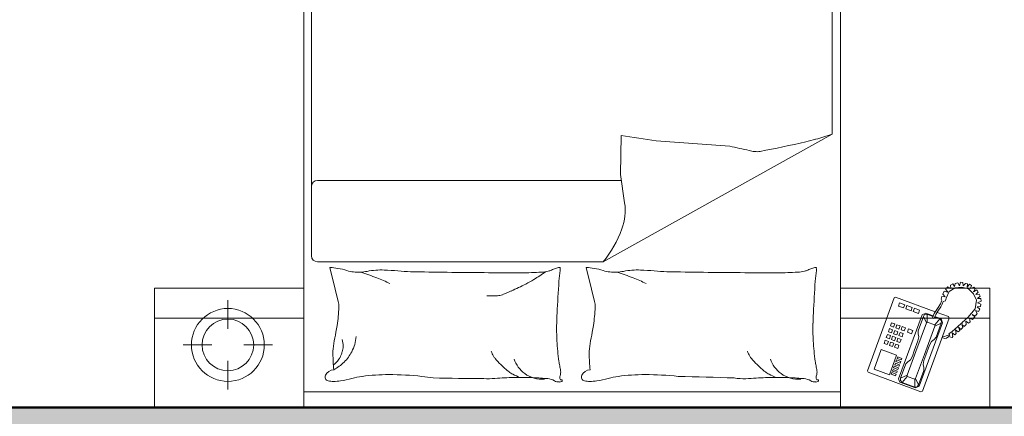
# Model space of a CAD drawing. Units: inches. Extents: x -7 to 1228, y -146 to 1091.
# Tile 60 of 88: x 429 to 531, y 573 to 614. Entities that reach past the tile are written whole.
import ezdxf

# ---------------------------------------------------------------- set-up
doc = ezdxf.new("R2010")
doc.units = ezdxf.units.IN
for name, color, linetype, lineweight in [('A-FURN', 8, 'Continuous', 18), ('A-WALL', 7, 'Continuous', 50), ('A-WALL-PATT', 251, 'Continuous', 13)]:
    doc.layers.add(name, color=color, linetype=linetype, lineweight=lineweight)
doc.styles.add('DIM_FONT', font='SIMPLEX.shx', dxfattribs={"width": 0.8})

# ---------------------------------------------------------------- blocks, each defined once
blk = doc.blocks.new('A$C4F634EDD')
for p, q in [((0, 2.6295), (0, 2.2295)), ((0.5, 2.6295), (0, 2.6295)), ((0.5, 2.6295), (2.3, 2.6295)), ((0.5, 0.5295), (0.5, 2.6295)), ((0.5, 2.2295), (0.5, 2.6295)), ((2.3, 2.6295), (2.3, 0.5295)), ((2.3, 2.6295), (2.8, 2.6295)), ((2.3, 2.2295), (2.3, 2.6295)), ((2.8, 2.6295), (2.8, 2.2295)), ((0.5, 2.5771), (2.3, 2.5771)), ((2.392, 2.5115), (2.5692, 2.5765)), ((2.5692, 2.5765), (2.574, 2.5743)), ((0.2457, 2.5697), (0.2457, 2.4733)), ((2.4946, 2.5331), (2.4985, 2.5445)), ((2.4985, 2.5445), (2.5516, 2.564)), ((2.5062, 2.5454), (2.5004, 2.5392)), ((2.5062, 2.5454), (2.5487, 2.561)), ((2.5235, 2.5256), (2.5062, 2.5454)), ((2.5483, 2.5347), (2.5487, 2.561)), ((2.5487, 2.561), (2.5571, 2.56)), ((2.5615, 2.5536), (2.5514, 2.5318)), ((2.5516, 2.564), (2.5637, 2.5584)), ((2.5571, 2.56), (2.5615, 2.5536)), ((2.5615, 2.5536), (2.5791, 2.5058)), ((2.5637, 2.5584), (2.6418, 2.3458)), ((2.574, 2.5743), (2.6638, 2.3298)), ((2.3898, 2.5066), (2.392, 2.5115)), ((2.412, 2.5007), (2.4634, 2.5196)), ((2.4634, 2.5196), (2.4875, 2.454)), ((2.4842, 2.5232), (2.47, 2.518)), ((2.47, 2.518), (2.472, 2.5127)), ((2.472, 2.5127), (2.4862, 2.5179)), ((2.4881, 2.5126), (2.4739, 2.5074)), ((2.4862, 2.5179), (2.4842, 2.5232)), ((2.4901, 2.5073), (2.4881, 2.5126)), ((2.5734, 2.3187), (2.4946, 2.5331)), ((2.5004, 2.5392), (2.5013, 2.5315)), ((2.5013, 2.5315), (2.5188, 2.4836)), ((2.5013, 2.5315), (2.5231, 2.5214)), ((2.5231, 2.5214), (2.5235, 2.5256)), ((2.5523, 2.4417), (2.5231, 2.5214)), ((2.5483, 2.5347), (2.5235, 2.5256)), ((2.5514, 2.5318), (2.5483, 2.5347)), ((2.5807, 2.4521), (2.5514, 2.5318)), ((2.4795, 2.2621), (2.3898, 2.5066)), ((2.4361, 2.4352), (2.412, 2.5007)), ((2.4739, 2.5074), (2.4759, 2.502)), ((2.4759, 2.502), (2.4901, 2.5073)), ((2.492, 2.5019), (2.4778, 2.4967)), ((2.4778, 2.4967), (2.4798, 2.4914)), ((2.4798, 2.4914), (2.494, 2.4966)), ((2.4959, 2.4913), (2.4817, 2.4861)), ((2.4817, 2.4861), (2.4837, 2.4808)), ((2.4837, 2.4808), (2.4979, 2.486)), ((2.4998, 2.4807), (2.4856, 2.4755)), ((2.494, 2.4966), (2.492, 2.5019)), ((2.4979, 2.486), (2.4959, 2.4913)), ((2.5018, 2.4754), (2.4998, 2.4807)), ((2.5188, 2.4836), (2.5256, 2.4761)), ((2.5256, 2.4761), (2.5342, 2.4692)), ((2.5788, 2.4956), (2.5767, 2.4848)), ((2.5767, 2.4848), (2.5795, 2.4717)), ((2.5791, 2.5058), (2.5788, 2.4956)), ((2.4875, 2.454), (2.4361, 2.4352)), ((2.4856, 2.4755), (2.4876, 2.4702)), ((2.4876, 2.4702), (2.5018, 2.4754)), ((2.5037, 2.47), (2.4895, 2.4648)), ((2.4895, 2.4648), (2.4915, 2.4595)), ((2.4915, 2.4595), (2.5057, 2.4647)), ((2.5057, 2.4647), (2.5037, 2.47)), ((2.5342, 2.4692), (2.5405, 2.4574)), ((2.5405, 2.4574), (2.547, 2.4397)), ((2.5795, 2.4717), (2.586, 2.454)), ((2.5807, 2.4521), (2.6158, 2.3564)), ((2.5984, 2.4204), (2.586, 2.454)), ((0.0957, 2.4197), (0.192, 2.4197)), ((0.2994, 2.4197), (0.3957, 2.4197)), ((2.4457, 2.4146), (2.4563, 2.4185)), ((2.4496, 2.4039), (2.4457, 2.4146)), ((2.4563, 2.4185), (2.4602, 2.4078)), ((2.4634, 2.4211), (2.474, 2.425)), ((2.4673, 2.4104), (2.4634, 2.4211)), ((2.4779, 2.4143), (2.4673, 2.4104)), ((2.474, 2.425), (2.4779, 2.4143)), ((2.4811, 2.4276), (2.4917, 2.4315)), ((2.485, 2.4169), (2.4811, 2.4276)), ((2.4956, 2.4208), (2.485, 2.4169)), ((2.4883, 2.4081), (2.4989, 2.412)), ((2.4917, 2.4315), (2.4956, 2.4208)), ((2.4989, 2.412), (2.5028, 2.4014)), ((2.5594, 2.4061), (2.547, 2.4397)), ((2.5523, 2.4417), (2.5875, 2.346)), ((2.6047, 2.4086), (2.5984, 2.4204)), ((2.4602, 2.4078), (2.4496, 2.4039)), ((2.4528, 2.3951), (2.4635, 2.399)), ((2.4567, 2.3844), (2.4528, 2.3951)), ((2.4674, 2.3883), (2.4567, 2.3844)), ((2.46, 2.3756), (2.4706, 2.3795)), ((2.4635, 2.399), (2.4674, 2.3883)), ((2.4706, 2.4016), (2.4812, 2.4055)), ((2.4745, 2.3909), (2.4706, 2.4016)), ((2.4706, 2.3795), (2.4745, 2.3689)), ((2.4851, 2.3949), (2.4745, 2.3909)), ((2.4777, 2.3821), (2.4883, 2.386)), ((2.4816, 2.3715), (2.4777, 2.3821)), ((2.4812, 2.4055), (2.4851, 2.3949)), ((2.4922, 2.3975), (2.4883, 2.4081)), ((2.4883, 2.386), (2.4922, 2.3754)), ((2.5028, 2.4014), (2.4922, 2.3975)), ((2.4954, 2.3886), (2.5061, 2.3925)), ((2.4993, 2.378), (2.4954, 2.3886)), ((2.51, 2.3819), (2.4993, 2.378)), ((2.5061, 2.3925), (2.51, 2.3819)), ((2.5238, 2.3769), (2.538, 2.3821)), ((2.5277, 2.3663), (2.5238, 2.3769)), ((2.538, 2.3821), (2.5419, 2.3715)), ((2.5622, 2.393), (2.5594, 2.4061)), ((2.5598, 2.372), (2.5601, 2.3822)), ((2.5601, 2.3822), (2.5622, 2.393)), ((2.6133, 2.4017), (2.6047, 2.4086)), ((2.6201, 2.3941), (2.6133, 2.4017)), ((2.6376, 2.3463), (2.6201, 2.3941)), ((2.6499, 2.3979), (2.6397, 2.3953)), ((2.6417, 2.39), (2.6488, 2.391)), ((2.6488, 2.391), (2.6538, 2.3895)), ((2.6551, 2.397), (2.6499, 2.3979)), ((2.6538, 2.3895), (2.6596, 2.388)), ((2.6627, 2.392), (2.6551, 2.397)), ((2.6596, 2.388), (2.6626, 2.3867)), ((2.6626, 2.3867), (2.6662, 2.388)), ((2.6692, 2.394), (2.6627, 2.392)), ((2.6662, 2.388), (2.6632, 2.3828)), ((2.6632, 2.3828), (2.6736, 2.3744)), ((2.6736, 2.3944), (2.6692, 2.394)), ((2.6765, 2.391), (2.6736, 2.3944)), ((2.6742, 2.3795), (2.6765, 2.391)), ((2.6824, 2.3858), (2.6742, 2.3795)), ((2.6873, 2.3815), (2.6824, 2.3858)), ((2.6853, 2.369), (2.6873, 2.3815)), ((0.2457, 2.366), (0.2457, 2.2697)), ((2.4639, 2.365), (2.46, 2.3756)), ((2.4745, 2.3689), (2.4639, 2.365)), ((2.4672, 2.3561), (2.4778, 2.36)), ((2.4711, 2.3455), (2.4672, 2.3561)), ((2.4817, 2.3494), (2.4711, 2.3455)), ((2.4778, 2.36), (2.4817, 2.3494)), ((2.4922, 2.3754), (2.4816, 2.3715)), ((2.4849, 2.3626), (2.4955, 2.3665)), ((2.4888, 2.352), (2.4849, 2.3626)), ((2.4994, 2.3559), (2.4888, 2.352)), ((2.4955, 2.3665), (2.4994, 2.3559)), ((2.5026, 2.3691), (2.5132, 2.373)), ((2.5065, 2.3585), (2.5026, 2.3691)), ((2.5171, 2.3624), (2.5065, 2.3585)), ((2.5132, 2.373), (2.5171, 2.3624)), ((2.5419, 2.3715), (2.5277, 2.3663)), ((2.5774, 2.3242), (2.5598, 2.372)), ((2.5774, 2.3242), (2.5875, 2.346)), ((2.5875, 2.346), (2.5905, 2.3431)), ((2.6154, 2.3522), (2.5905, 2.3431)), ((2.6158, 2.3564), (2.6154, 2.3522)), ((2.6154, 2.3522), (2.6327, 2.3324)), ((2.6376, 2.3463), (2.6158, 2.3564)), ((2.6418, 2.3458), (2.6369, 2.332)), ((2.6385, 2.3386), (2.6376, 2.3463)), ((2.6736, 2.3744), (2.6922, 2.3593)), ((2.6946, 2.376), (2.6853, 2.369)), ((2.6922, 2.3593), (2.7051, 2.3473)), ((2.6995, 2.3713), (2.6946, 2.376)), ((2.695, 2.3603), (2.6995, 2.3713)), ((2.7031, 2.3682), (2.695, 2.3603)), ((2.7096, 2.3616), (2.7031, 2.3682)), ((2.7051, 2.3473), (2.7079, 2.3475)), ((2.7062, 2.351), (2.7096, 2.3616)), ((2.7147, 2.3578), (2.7062, 2.351)), ((2.7079, 2.3475), (2.7079, 2.3443)), ((2.7079, 2.3443), (2.727, 2.3277)), ((2.7214, 2.3517), (2.7147, 2.3578)), ((2.7196, 2.34), (2.7214, 2.3517)), ((2.7286, 2.3466), (2.7196, 2.34)), ((2.7346, 2.3423), (2.7286, 2.3466)), ((0, 2.3301), (0.5, 2.3301)), ((2.8, 2.3301), (2.3, 2.3301)), ((2.561, 2.3141), (2.5433, 2.3076)), ((2.5649, 2.3035), (2.561, 2.3141)), ((2.5855, 2.3131), (2.5734, 2.3187)), ((2.5818, 2.3178), (2.5774, 2.3242)), ((2.5901, 2.3168), (2.5818, 2.3178)), ((2.6104, 2.3222), (2.5855, 2.3131)), ((2.5905, 2.3431), (2.5901, 2.3168)), ((2.5901, 2.3168), (2.6097, 2.324)), ((2.613, 2.3312), (2.6077, 2.3293)), ((2.6077, 2.3293), (2.6135, 2.3141)), ((2.6192, 2.3174), (2.613, 2.3312)), ((2.6135, 2.3141), (2.6244, 2.2977)), ((2.6153, 2.3261), (2.6327, 2.3324)), ((2.6369, 2.332), (2.6161, 2.3243)), ((2.626, 2.3069), (2.6192, 2.3174)), ((2.6616, 2.3249), (2.6234, 2.3109)), ((2.6327, 2.3324), (2.6385, 2.3386)), ((2.6638, 2.3298), (2.6616, 2.3249)), ((2.727, 2.3277), (2.7512, 2.2983)), ((2.732, 2.3295), (2.7346, 2.3423)), ((2.7423, 2.3345), (2.732, 2.3295)), ((2.7406, 2.3172), (2.7495, 2.325)), ((2.7519, 2.3218), (2.7406, 2.3172)), ((2.7495, 2.325), (2.7423, 2.3345)), ((2.7575, 2.3144), (2.7519, 2.3218)), ((2.7526, 2.3045), (2.7575, 2.3144)), ((2.6172, 2.3086), (2.4844, 2.2599)), ((2.5114, 2.2959), (2.4936, 2.2894)), ((2.4936, 2.2894), (2.4976, 2.2788)), ((2.4976, 2.2788), (2.5153, 2.2853)), ((2.5153, 2.2853), (2.5114, 2.2959)), ((2.5362, 2.305), (2.5185, 2.2985)), ((2.5185, 2.2985), (2.5224, 2.2879)), ((2.5224, 2.2879), (2.5401, 2.2944)), ((2.5401, 2.2944), (2.5362, 2.305)), ((2.5433, 2.3076), (2.5472, 2.297)), ((2.5472, 2.297), (2.5649, 2.3035)), ((2.6244, 2.2977), (2.6349, 2.2825)), ((2.6365, 2.2916), (2.626, 2.3069)), ((2.6349, 2.2825), (2.638, 2.273)), ((2.6407, 2.2834), (2.6365, 2.2916)), ((2.6438, 2.2739), (2.6407, 2.2834)), ((2.7512, 2.2983), (2.756, 2.2695)), ((2.7622, 2.308), (2.7526, 2.3045)), ((2.7574, 2.2924), (2.7673, 2.2997)), ((2.7687, 2.2905), (2.7574, 2.2924)), ((2.7587, 2.279), (2.7699, 2.2828)), ((2.7708, 2.2725), (2.7587, 2.279)), ((2.7673, 2.2997), (2.7622, 2.308)), ((2.7699, 2.2828), (2.7687, 2.2905)), ((0.5953, 2.1912), (0.616, 2.2738)), ((1.4546, 2.1912), (1.4752, 2.2738)), ((2.4844, 2.2599), (2.4795, 2.2621)), ((2.6399, 2.2712), (2.6374, 2.2659)), ((2.6374, 2.2659), (2.6398, 2.257)), ((2.638, 2.273), (2.6399, 2.2712)), ((2.6398, 2.257), (2.6509, 2.259)), ((2.6509, 2.259), (2.6431, 2.2492)), ((2.6431, 2.2492), (2.6473, 2.2398)), ((2.6519, 2.2716), (2.6438, 2.2739)), ((2.6535, 2.2628), (2.6519, 2.2716)), ((2.6636, 2.2409), (2.6535, 2.2628)), ((2.7459, 2.2483), (2.7284, 2.2317)), ((2.756, 2.2695), (2.7459, 2.2483)), ((2.7529, 2.2505), (2.7645, 2.2498)), ((2.7607, 2.2424), (2.7529, 2.2505)), ((2.759, 2.2637), (2.7706, 2.2643)), ((2.7676, 2.2559), (2.759, 2.2637)), ((2.7645, 2.2498), (2.7676, 2.2559)), ((2.7706, 2.2643), (2.7708, 2.2725)), ((0, 2.2295), (0.5, 2.2295)), ((2.8, 2.2295), (2.3, 2.2295)), ((2.6473, 2.2398), (2.6592, 2.2429)), ((2.6592, 2.2429), (2.6521, 2.2314)), ((2.6521, 2.2314), (2.6598, 2.2248)), ((2.6598, 2.2248), (2.6697, 2.2309)), ((2.6836, 2.2287), (2.6636, 2.2409)), ((2.6697, 2.2309), (2.6684, 2.219)), ((2.6684, 2.219), (2.6761, 2.2145)), ((2.6761, 2.2145), (2.6821, 2.2237)), ((2.6821, 2.2237), (2.6843, 2.2135)), ((2.7063, 2.2256), (2.6836, 2.2287)), ((2.6843, 2.2135), (2.6927, 2.2117)), ((2.6927, 2.2117), (2.6986, 2.222)), ((2.6986, 2.222), (2.7019, 2.2098)), ((2.7284, 2.2317), (2.7063, 2.2256)), ((2.7102, 2.2104), (2.7113, 2.2218)), ((2.7113, 2.2218), (2.7192, 2.2137)), ((2.7192, 2.2137), (2.7255, 2.2152)), ((2.7255, 2.2152), (2.7242, 2.2265)), ((2.7242, 2.2265), (2.7324, 2.2165)), ((2.7324, 2.2165), (2.7386, 2.2208)), ((2.7386, 2.2208), (2.7354, 2.2306)), ((2.7354, 2.2306), (2.7462, 2.2264)), ((2.7509, 2.2314), (2.7459, 2.2418)), ((2.7459, 2.2418), (2.7568, 2.2352)), ((2.7462, 2.2264), (2.7509, 2.2314)), ((2.7568, 2.2352), (2.7607, 2.2424)), ((0.5878, 2.1612), (0.5953, 2.1912)), ((1.4471, 2.1612), (1.4546, 2.1912)), ((2.7019, 2.2098), (2.7102, 2.2104)), ((0.5258, 2.121), (0.5258, 0.5617)), ((1.5035, 2.141), (0.5458, 2.141)), ((1.5035, 2.141), (2.2716, 1.7136)), ((1.576, 1.9433), (1.5624, 1.8479)), ((0.5458, 1.8684), (1.5653, 1.8684)), ((1.5624, 1.8479), (1.5641, 1.7178)), ((2.2716, 0.5617), (2.2716, 1.7136))]:
    blk.add_line(p, q)
for radius in [0.1222, 0.0865]:
    blk.add_circle((0.2457, 2.4197), radius)
for centre, radius, start, end in [((0.5999, 2.4516), 0.0904, 90, 101.2724), ((0.5999, 2.3808), 0.1611, 81.5628, 90), ((1.3554, 2.5152), 0.0289, 85.6975, 120.6513), ((1.3556, 2.519), 0.0251, 68.2117, 85.6975), ((1.3637, 2.5391), 0.00342, 19.564, 68.2117), ((1.4591, 2.4516), 0.0904, 90, 101.2724), ((1.4591, 2.3808), 0.1611, 81.5628, 90), ((2.2146, 2.5152), 0.0289, 85.6975, 120.6513), ((2.2149, 2.519), 0.0251, 68.2117, 85.6975), ((2.2229, 2.5391), 0.00342, 19.564, 68.2117), ((0.5848, 2.5274), 0.0131, 101.2724, 206.5805), ((0.6036, 2.5368), 0.0342, 206.5805, 265.5998), ((0.5788, 2.2388), 0.3048, 74.256, 81.5628), ((0.7272, 2.7653), 0.2422, 254.256, 262.4531), ((0.7851, 3.2019), 0.6827, 262.4531, 270), ((0.7851, 3.5682), 1.049, 270, 276.0867), ((0.8402, 3.0514), 0.5293, 276.0867, 280.1899), ((1.1602, -8.1346), 10.6675, 90.30153, 91.21582), ((1.1169, 2.2433), 0.2897, 85.1982, 92.5386), ((1.2142, 3.4021), 0.8732, 265.1982, 269.4243), ((1.4317, 2.2032), 0.3916, 128.3886, 133.8115), ((1.2362, 2.45), 0.0768, 117.2396, 128.3886), ((1.3082, 2.3102), 0.234, 110.8603, 117.2396), ((1.2204, 4.0232), 1.4943, 269.4243, 271.9079), ((1.2995, 2.4357), 0.0992, 126.0864, 143.8234), ((1.2995, 2.4357), 0.0992, 105.9352, 126.0864), ((1.2429, 3.3501), 0.8208, 271.9079, 275.2592), ((1.2995, 2.4357), 0.0992, 85.7841, 105.9352), ((1.3132, 2.5864), 0.0539, 275.2592, 300.6513), ((1.3739, 2.5288), 0.0156, 158.0096, 201.421), ((1.3634, 2.533), 0.00428, 78.1069, 158.0096), ((1.3288, 2.5111), 0.0328, 351.8665, 21.421), ((1.3647, 2.5395), 0.00232, 258.1069, 19.564), ((1.444, 2.5274), 0.0131, 101.2724, 206.5805), ((1.4628, 2.5368), 0.0342, 206.5805, 265.5998), ((1.438, 2.2388), 0.3048, 74.256, 81.5628), ((1.5865, 2.7653), 0.2422, 254.256, 262.4531), ((1.6443, 3.2019), 0.6827, 262.4531, 270), ((1.6443, 3.5682), 1.049, 270, 276.0867), ((1.4785, 15.4878), 12.9656, 271.22425, 272.05324), ((1.97, 2.3805), 0.1524, 92.5386, 100.1899), ((1.9761, 2.2433), 0.2897, 85.1982, 92.5386), ((2.0734, 3.4021), 0.8732, 265.1982, 269.4243), ((2.291, 2.2032), 0.3916, 128.3886, 133.8115), ((2.0954, 2.45), 0.0768, 117.2396, 128.3886), ((2.1674, 2.3102), 0.234, 110.8603, 117.2396), ((2.0797, 4.0232), 1.4943, 269.4243, 271.9079), ((2.1588, 2.4357), 0.0992, 126.0864, 143.8234), ((2.1588, 2.4357), 0.0992, 105.9352, 126.0864), ((2.1021, 3.3501), 0.8208, 271.9079, 275.2592), ((2.1588, 2.4357), 0.0992, 85.7841, 105.9352), ((2.1724, 2.5864), 0.0539, 275.2592, 300.6513), ((2.2331, 2.5288), 0.0156, 158.0096, 201.421), ((2.2226, 2.533), 0.00428, 78.1069, 158.0096), ((2.1881, 2.5111), 0.0328, 351.8665, 21.421), ((2.224, 2.5395), 0.00232, 258.1069, 19.564), ((1.0898, 2.4496), 0.4918, 173.7676, 180), ((0.5462, 2.4142), 0.0899, 41.4429, 53.7359), ((0.5368, 2.3783), 0.1399, 45.0976, 62.7964), ((0.5368, 2.3783), 0.1399, 27.3988, 45.0976), ((1.3165, 2.3233), 0.2252, 133.8115, 140.9651), ((1.2995, 2.4357), 0.0992, 143.8234, 161.5603), ((1.5522, 2.448), 0.1983, 167.8905, 172.3191), ((1.1177, 2.5413), 0.246, 347.8905, 351.8665), ((1.949, 2.4496), 0.4918, 173.7676, 180), ((2.1757, 2.3233), 0.2252, 133.8115, 140.9651), ((2.1588, 2.4357), 0.0992, 143.8234, 161.5603), ((2.4114, 2.448), 0.1983, 167.8905, 172.3191), ((1.977, 2.5413), 0.246, 347.8905, 351.8665), ((0.8019, 2.4496), 0.204, 180, 189.6844), ((0.5741, 2.4389), 0.0526, 25.3551, 41.4429), ((0.4851, 2.3967), 0.1511, 21.8149, 25.3551), ((0.4345, 2.3765), 0.2056, 18.7799, 21.8149), ((1.3127, 2.3625), 0.2002, 151.6832, 156.9972), ((1.1799, 2.4341), 0.0493, 140.9651, 151.6832), ((2.2605, 2.3525), 0.9131, 172.3191, 176.6313), ((1.6611, 2.4496), 0.204, 180, 189.6844), ((2.1719, 2.3625), 0.2002, 151.6832, 156.9972), ((2.0391, 2.4341), 0.0493, 140.9651, 151.6832), ((3.1198, 2.3525), 0.9131, 172.3191, 176.6313), ((1.4703, 2.5637), 0.882, 189.6844, 192.1984), ((0.576, 2.4246), 0.0562, 0, 18.7799), ((0.5406, 2.4246), 0.0915, 345.3149, 0), ((0.5368, 2.3783), 0.1399, 16.515, 27.3988), ((0.5368, 2.3783), 0.1399, 5.6311, 16.515), ((2.3295, 2.5637), 0.882, 189.6844, 192.1984), ((0.2982, 2.3103), 0.3171, 8.0051, 12.1984), ((2.0266, 2.3663), 0.6787, 176.6313, 181.6331), ((1.1575, 2.3103), 0.3171, 8.0051, 12.1984), ((2.8858, 2.3663), 0.6787, 176.6313, 181.6331), ((-0.0401, 2.2627), 0.6588, 2.6649, 8.0051), ((2.7128, 2.3859), 1.3652, 181.6331, 183.055), ((0.8191, 2.2627), 0.6588, 2.6649, 8.0051), ((3.5721, 2.3859), 1.3652, 181.6331, 183.055), ((14.9657, 3.0398), 13.6356, 183.05496, 183.50486), ((15.8249, 3.0398), 13.6356, 183.05496, 183.50486), ((0.5503, 2.2902), 0.0677, 345.9548, 2.6649), ((1.4096, 2.2902), 0.0677, 345.9548, 2.6649), ((1.1303, 1.9835), 0.2721, 85.9172, 93.5552), ((1.1455, 2.197), 0.058, 69.3257, 85.9172), ((0.9871, 1.7772), 0.5066, 65.6735, 69.3257), ((0.473, 2.8815), 0.7387, 293.4844, 295.3111), ((0.6058, 0.9338), 1.4323, 63.5015, 65.6735), ((1.1054, 1.9358), 0.3126, 57.865, 63.5015), ((1.3322, 2.8815), 0.7387, 293.4844, 295.3111), ((0.473, 2.8815), 0.7387, 287.1982, 289.428), ((0.473, 2.8815), 0.7387, 289.428, 291.6577), ((0.473, 2.8815), 0.7387, 291.6577, 293.4844), ((0.8841, 1.5835), 0.7286, 54.1737, 57.865), ((1.6762, 2.2258), 0.3212, 183.5049, 189.9984), ((1.3322, 2.8815), 0.7387, 287.1982, 289.428), ((1.3322, 2.8815), 0.7387, 289.428, 291.6577), ((1.3322, 2.8815), 0.7387, 291.6577, 293.4844), ((2.5355, 2.2258), 0.3212, 183.5049, 189.9984), ((0.5887, 2.1609), 0.000917, 165.9551, 274.0829), ((0.5695, 2.4301), 0.2708, 274.0829, 279.4841), ((0.5763, 2.3896), 0.2297, 279.4841, 287.3864), ((0.6807, 2.0561), 0.1197, 96.4341, 107.3864), ((0.6836, 2.0301), 0.1459, 78.4414, 96.4341), ((0.759, 2.3985), 0.2301, 258.4414, 272.7491), ((0.7026, 3.5718), 1.4048, 272.7491, 274.6176), ((0.9136, 0.9591), 1.2165, 92.6096, 94.6176), ((1.2501, -19.8405), 22.0183, 90.37908, 91.01965), ((1.2012, -3.5404), 5.7185, 89.7135, 90.9704), ((1.224, 1.0141), 1.164, 86.426, 89.7135), ((1.2875, 2.0302), 0.1459, 77.131, 86.426), ((1.3099, 2.1283), 0.0453, 62.7159, 77.131), ((1.3658, 2.2367), 0.0767, 242.7159, 253.7788), ((1.3688, 2.247), 0.0875, 253.7788, 262.8796), ((1.3581, 2.1615), 0.00132, 262.8796, 343.3022), ((1.3409, 2.1667), 0.0193, 343.3022, 9.9984), ((1.448, 2.1609), 0.000917, 165.9551, 274.0829), ((1.4288, 2.4301), 0.2708, 274.0829, 279.4841), ((1.4355, 2.3896), 0.2297, 279.4841, 287.3864), ((1.5399, 2.0561), 0.1197, 96.4341, 107.3864), ((1.5429, 2.0301), 0.1459, 78.4414, 96.4341), ((1.6182, 2.3985), 0.2301, 258.4414, 272.7491), ((1.5619, 3.5718), 1.4048, 272.7491, 274.6176), ((1.7729, 0.9591), 1.2165, 92.6096, 94.6176), ((2.1093, -19.8405), 22.0183, 90.37908, 91.01965), ((2.0605, -3.5404), 5.7185, 89.7135, 90.9704), ((2.0833, 1.0141), 1.164, 86.426, 89.7135), ((2.1467, 2.0302), 0.1459, 77.131, 86.426), ((2.1691, 2.1283), 0.0453, 62.7159, 77.131), ((2.2251, 2.2367), 0.0767, 242.7159, 253.7788), ((2.2281, 2.247), 0.0875, 253.7788, 262.8796), ((2.2174, 2.1615), 0.00132, 262.8796, 343.3022), ((2.2001, 2.1667), 0.0193, 343.3022, 9.9984), ((0.5458, 2.121), 0.02, 90, 180), ((1.2147, 1.9017), 0.3751, 20.1488, 39.6445), ((1.3977, 1.9688), 0.1801, 351.8644, 20.1488), ((0.5458, 1.8884), 0.02, 180, 270), ((0.6102, 18.0525), 16.3521, 273.75703, 274.62393), ((1.4194, 4.2174), 2.5158, 281.6741, 283.1904), ((2.0378, 1.5789), 0.1942, 97.7304, 103.1904), ((2.0195, 1.7137), 0.0581, 79.2724, 97.7304), ((1.2737, -2.2227), 4.0646, 77.0745, 79.2724), ((1.0582, 5.4638), 3.7801, 277.692, 279.495), ((2.0359, 1.0981), 0.6574, 74.0648, 77.0745), ((1.7125, -0.0344), 1.8351, 72.2636, 74.0648)]:
    blk.add_arc(centre, radius, start, end)
at = {"style": 'DIM_FONT', "width": 0.8, "flags": 9}
for tag, p in [('YSIZE', (0.5, 2.6295)), ('XSIZE', (0.5, 2.6295)), ('XSIZE', (2.2985, 2.6295)), ('YSIZE', (2.2985, 2.6295))]:
    blk.add_attdef(tag, p, '', height=0.0005, dxfattribs=at)

msp = doc.modelspace()

# ---------------------------------------------------------------- hatches: boundary and pattern name
at = {"layer": 'A-WALL-PATT'}
h = msp.add_hatch(color=256, dxfattribs=at)
h.dxf.hatch_style = 1
h.paths.add_polyline_path([(69, 568), (60, 568), (60, 493), (63.29, 493), (69, 493)])
h.paths.add_polyline_path([(69, 662.41), (60, 662.41), (60, 586), (69, 586)], flags=17)
h.paths.add_polyline_path([(69, 723), (184, 723), (184, 734), (179, 734), (179, 728), (69, 728), (69, 741.62), (60, 741.62), (60, 698.41), (69, 698.41)], flags=17)
h.paths.add_polyline_path([(69, 782), (231, 782), (231, 728), (231, 723), (231, 586), (236, 586), (236, 787), (69, 787), (69, 800.13), (60, 800.13), (60, 765.62), (69, 765.62)])
h.paths.add_polyline_path([(184, 842), (189, 842), (189, 848), (173, 848), (173, 842), (179, 842), (179, 787), (184, 787)])
h.paths.add_polyline_path([(118.22, 69), (69, 69), (69, 60), (118.22, 60)])
h.paths.add_polyline_path([(227, 69), (154.22, 69), (154.22, 60), (227, 60)])
h.paths.add_polyline_path([(236, 60), (232.71, 60), (227, 60), (227, 36), (236, 36)])
h.paths.add_polyline_path([(389, 60), (380, 60), (380, 36), (389, 36)])
h.paths.add_polyline_path([(384, 181), (380, 181), (380, 115), (380, 78), (384, 78)])
h.paths.add_polyline_path([(380, 115), (334.55, 115), (334.55, 109), (380, 109)])
h.paths.add_polyline_path([(274.55, 115), (236, 115), (236, 201), (232.71, 201), (231, 201), (231, 78), (236, 78), (236, 109), (274.55, 109)])
h.paths.add_polyline_path([(69, 123), (60, 123), (60, 78), (69, 78)])
h.paths.add_polyline_path([(69, 201), (60, 201), (60, 159), (69, 159)])
h.paths.add_polyline_path([(143, 219), (69, 219), (69, 213), (143, 213)], flags=17)
h.paths.add_polyline_path([(189, 219), (184, 219), (184, 274), (231, 274), (231, 219), (236, 219), (236, 279), (184, 279), (184, 297), (179, 297), (179, 279), (69, 279), (69, 290.91), (60, 290.91), (60, 262.18), (69, 262.18), (69, 274), (179, 274), (179, 219), (173, 219), (173, 213), (189, 213)])
h.paths.add_polyline_path([(69, 238.18), (60, 238.18), (60, 219), (69, 219)], flags=17)
h.paths.add_polyline_path([(69, 333), (60, 333), (60, 314.91), (69, 314.91), (69, 316.96)])
h.paths.add_polyline_path([(190, 338), (184, 338), (69, 338), (69, 333), (179, 333), (179, 327), (184, 327), (184, 333.02), (190, 333.05)])
h.paths.add_polyline_path([(69, 386.81), (60, 386.81), (60, 351), (69, 351)])
h.paths.add_polyline_path([(69, 475), (60, 475), (60, 422.81), (69, 422.81)])
h.paths.add_polyline_path([(236, 475), (231, 475), (231, 351.24), (236, 351.24)])
h.paths.add_polyline_path([(384, 475), (380, 475), (380, 362), (384, 362)])
h.paths.add_polyline_path([(547, 307), (439, 307), (439, 356), (445, 356), (445, 362), (433, 362), (433, 307), (380, 307), (380, 244), (380, 241), (384, 241), (384, 301), (433, 301), (433, 277), (439, 277), (439, 301), (547, 301)])
h.paths.add_polyline_path([(547, 241), (439, 241), (439, 247), (433, 247), (433, 235), (547, 235)])
h.paths.add_polyline_path([(450, 69), (440.29, 69), (424.89, 69), (389, 69), (389, 60), (450, 60)])
h.paths.add_polyline_path([(547, 69), (486, 69), (486, 60), (547, 60)])
h.paths.add_polyline_path([(556, 148.27), (547, 148.27), (547, 78), (556, 78)])
h.paths.add_polyline_path([(556, 223), (547, 223), (547, 195), (547, 184.27), (556, 184.27)])
h.paths.add_polyline_path([(556, 311.19), (547, 311.19), (547, 273.08), (556, 273.08)])
h.paths.add_polyline_path([(556, 344), (552.71, 344), (547, 344), (547, 335.19), (556, 335.19)])
h.paths.add_polyline_path([(556, 249.08), (547, 249.08), (547, 241), (556, 241)])
h.paths.add_polyline_path([(547, 362), (475, 362), (475, 356), (547, 356)], flags=0)
h.paths.add_polyline_path([(556, 399.62), (547, 399.62), (547, 362), (556, 362)])
h.paths.add_polyline_path([(556, 475), (547, 475), (547, 435.62), (556, 435.62)])
h.paths.add_polyline_path([(547, 493), (389, 493), (389, 487), (547, 487)])
h.paths.add_polyline_path([(380, 493), (278, 493), (278, 487), (380, 487)])
h.paths.add_polyline_path([(227, 493), (69, 493), (69, 487), (227, 487)])
h.paths.add_polyline_path([(643, 122.44), (634, 122.44), (634, 78), (643, 78)])
h.paths.add_polyline_path([(702.5, 69), (692.79, 69), (677.39, 69), (643, 69), (643, 60), (702.5, 60)])
h.paths.add_polyline_path([(798, 69), (738.5, 69), (738.5, 60), (798, 60)])
h.paths.add_polyline_path([(807, 60), (803.71, 60), (798, 60), (798, 36), (807, 36)])
h.paths.add_polyline_path([(807, 109), (846.75, 109), (846.75, 115), (807, 115), (807, 159), (802, 159), (802, 78), (807, 78)])
h.paths.add_polyline_path([(807, 201), (802, 201), (802, 195), (807, 195)])
h.paths.add_polyline_path([(643, 201), (634, 201), (634, 158.44), (643, 158.44)])
h.paths.add_polyline_path([(756, 225), (751, 225), (751, 219), (643, 219), (643, 213), (756, 213)])
h.paths.add_polyline_path([(643, 240.85), (634, 240.85), (634, 219), (643, 219)])
h.paths.add_polyline_path([(643, 274), (643, 288.63), (634, 288.63), (634, 264.85), (643, 264.85)])
h.paths.add_polyline_path([(802, 279), (756, 279), (756, 297), (751, 297), (751, 279), (643, 279), (643, 274), (751, 274), (751, 255), (756, 255), (756, 274), (802, 274)])
h.paths.add_polyline_path([(807, 333), (803.71, 333), (802, 333), (802, 279), (802, 274), (802, 219), (807, 219)])
h.paths.add_polyline_path([(956, 182), (951, 182), (951, 115), (906.75, 115), (906.75, 109), (951, 109), (951, 78), (956, 78)])
h.paths.add_polyline_path([(960, 60), (951, 60), (951, 36), (960, 36)])
h.paths.add_polyline_path([(1021, 69), (1005.78, 69), (960, 69), (960, 60), (1021, 60)])
h.paths.add_polyline_path([(956, 224), (951, 224), (951, 218), (956, 218)])
h.paths.add_polyline_path([(956, 302), (1004, 302), (1004, 278), (1010, 278), (1010, 302), (1118, 302), (1118, 290.81), (1127, 290.81), (1127, 326.97), (1118, 326.97), (1118, 320.97), (1118, 307), (1010, 307), (1010, 356), (1016, 356), (1016, 362), (1004, 362), (1004, 307), (951, 307), (951, 244), (951, 242), (954.29, 242), (956, 242)])
h.paths.add_polyline_path([(643, 333), (634, 333), (634, 312.63), (643, 312.63), (643, 316.96)])
h.paths.add_polyline_path([(756, 338), (643, 338), (643, 333), (751, 333), (751, 327), (756, 327)])
h.paths.add_polyline_path([(643, 388), (634, 388), (634, 351), (643, 351)])
h.paths.add_polyline_path([(807, 357), (802, 357), (802, 351), (807, 351)])
h.paths.add_polyline_path([(807, 475), (802, 475), (802, 393), (807, 393)])
h.paths.add_polyline_path([(643, 475), (634, 475), (634, 424), (643, 424)])
h.paths.add_polyline_path([(798, 493), (643, 493), (643, 487), (798, 487)])
h.paths.add_polyline_path([(634, 493), (556, 493), (556, 487), (634, 487)])
h.paths.add_polyline_path([(813, 493), (807, 493), (807, 487), (813, 487)])
h.paths.add_polyline_path([(951, 493), (849, 493), (849, 487), (951, 487)])
h.paths.add_polyline_path([(956, 484), (951, 484), (951, 374), (956, 374)])
h.paths.add_polyline_path([(1109, 493), (969, 493), (969, 487), (1109, 487)])
h.paths.add_polyline_path([(1127, 484), (1118, 484), (1118, 450.64), (1127, 450.64)])
h.paths.add_polyline_path([(1127, 414.64), (1118, 414.64), (1118, 365), (1127, 365)])
h.paths.add_polyline_path([(1109, 362), (1046, 362), (1046, 356), (1109, 356)], flags=17)
h.paths.add_polyline_path([(1127, 356), (1123.45, 356), (1118, 356), (1118, 350.97), (1127, 350.97)], flags=0)
h.paths.add_polyline_path([(1127, 266.81), (1118, 266.81), (1118, 262.36), (1118, 242), (1127, 242)], flags=17)
h.paths.add_polyline_path([(1118, 242), (1010, 242), (1010, 248), (1004, 248), (1004, 237), (1118, 237)])
h.paths.add_polyline_path([(1127, 224), (1118, 224), (1118, 170), (1127, 170)])
h.paths.add_polyline_path([(1127, 134), (1118, 134), (1118, 78), (1127, 78)])
h.paths.add_polyline_path([(1118, 69), (1057, 69), (1057, 60), (1118, 60)])
h.paths.add_polyline_path([(227, 571.55), (227, 574), (69, 574), (69, 568), (227, 568)])
h.paths.add_polyline_path([(380, 571.55), (380, 574), (278, 574), (278, 568), (380, 568)])
h.paths.add_polyline_path([(242, 574), (236, 574), (236, 568), (242, 568)])
h.paths.add_polyline_path([(547, 571.55), (547, 574), (389, 574), (389, 568), (547, 568)])
h.paths.add_polyline_path([(384, 733), (380, 733), (380, 586), (384, 586)])
h.paths.add_polyline_path([(556, 646), (634, 646), (634, 655), (547, 655), (547, 586), (556, 586)])
h.paths.add_polyline_path([(634, 574), (556, 574), (556, 568), (634, 568)])
h.paths.add_polyline_path([(643, 655), (634, 655), (634, 586), (643, 586)])
h.paths.add_polyline_path([(798, 574), (643, 574), (643, 568), (798, 568)])
h.paths.add_polyline_path([(643, 663.85), (634, 663.85), (634, 655), (643, 655)])
h.paths.add_polyline_path([(556, 676.97), (547, 676.97), (547, 655), (556, 655)])
h.paths.add_polyline_path([(556, 733), (547, 733), (547, 712.97), (556, 712.97)])
h.paths.add_polyline_path([(643, 710), (634, 710), (634, 699.85), (643, 699.85)])
h.paths.add_polyline_path([(807, 668), (802, 668), (802, 586), (807, 586)])
h.paths.add_polyline_path([(951, 574), (849, 574), (849, 568), (951, 568)])
h.paths.add_polyline_path([(956, 691), (951, 691), (951, 577), (956, 577)])
h.paths.add_polyline_path([(1109, 574), (969, 574), (969, 568), (1109, 568)])
h.paths.add_polyline_path([(1127, 643.4), (1118, 643.4), (1118, 577), (1127, 577)])
h.paths.add_polyline_path([(1127, 568), (1123.45, 568), (1118, 568), (1118, 493), (1127, 493)])
h.paths.add_polyline_path([(1127, 733), (1118, 733), (1118, 679.4), (1127, 679.4)])
h.paths.add_polyline_path([(1127, 777.35), (1118, 777.35), (1118, 770.04), (1118, 751), (1127, 751)], flags=17)
h.paths.add_polyline_path([(1118, 751), (1010, 751), (1010, 757), (1004, 757), (1004, 745), (1118, 745)])
h.paths.add_polyline_path([(956, 811), (1004, 811), (1004, 787), (1010, 787), (1010, 811), (1017.87, 811), (1017.87, 811.63, -0.414214), (1018.25, 812), (1031.98, 812, -0.414214), (1032.35, 811.63), (1032.35, 811), (1118, 811), (1118, 801.35), (1127, 801.35), (1127, 834.69), (1118, 834.69), (1118, 830.24), (1118, 817), (1010, 817), (1010, 866), (1016, 866), (1016, 872), (1004, 872), (1004, 817), (956, 817), (956, 866), (951, 866), (951, 751), (954.29, 751), (956, 751)])
h.paths.add_polyline_path([(1118, 872), (1046, 872), (1046, 866), (1118, 866)], flags=17)
h.paths.add_polyline_path([(1127, 924.71), (1118, 924.71), (1118, 884), (1127, 884)])
h.paths.add_polyline_path([(1127, 866), (1123.71, 866), (1118, 866), (1118, 858.69), (1127, 858.69)], flags=17)
h.paths.add_polyline_path([(956, 983), (951, 983), (951, 952), (807, 952), (807, 983), (802, 983), (802, 902), (807, 902), (807, 946), (951, 946), (951, 884), (956, 884)])
h.paths.add_polyline_path([(807, 842), (802, 842), (802, 787), (756, 787), (756, 806), (751, 806), (751, 787), (643, 787), (643, 782), (751, 782), (751, 764), (756, 764), (756, 782), (802, 782), (802, 728), (807, 728)])
h.paths.add_polyline_path([(756, 848), (643, 848), (643, 842), (751, 842), (751, 836), (756, 836)])
h.paths.add_polyline_path([(756, 734), (751, 734), (751, 728), (643, 728), (643, 723), (756, 723)])
h.paths.add_polyline_path([(643, 749.79), (634, 749.79), (634, 728), (637.29, 728), (643, 728)])
h.paths.add_polyline_path([(643, 805.41), (634, 805.41), (634, 773.79), (643, 773.79)])
h.paths.add_polyline_path([(643, 896.66), (634, 896.66), (634, 860), (637.29, 860), (643, 860)])
h.paths.add_polyline_path([(643, 842), (634, 842), (634, 829.41), (643, 829.41)])
h.paths.add_polyline_path([(643, 983), (634, 983), (634, 932.66), (643, 932.66)])
h.paths.add_polyline_path([(1127, 983), (1118, 983), (1118, 960.71), (1127, 960.71)])
h.paths.add_polyline_path([(1118, 1001), (1077.53, 1001), (1077.53, 992), (1118, 992)])
h.paths.add_polyline_path([(1041.53, 1001), (960, 1001), (960, 992), (1041.53, 992)])
h.paths.add_polyline_path([(960, 1025), (951, 1025), (951, 1001), (954.29, 1001), (960, 1001)])
h.paths.add_polyline_path([(807, 1025), (798, 1025), (798, 1001), (807, 1001)])
h.paths.add_polyline_path([(798, 1001), (738.5, 1001), (738.5, 992), (798, 992)])
h.paths.add_polyline_path([(702.5, 1001), (643, 1001), (643, 992), (702.5, 992)])
h.paths.add_polyline_path([(547, 1001), (499.11, 1001), (499.11, 992), (547, 992)])
h.paths.add_polyline_path([(463.11, 1001), (389, 1001), (389, 992), (463.11, 992)])
h.paths.add_polyline_path([(389, 1025), (380, 1025), (380, 1022), (380, 1001), (383.29, 1001), (389, 1001)])
h.paths.add_polyline_path([(236, 1025), (227, 1025), (227, 1001), (236, 1001)])
h.paths.add_polyline_path([(236, 983), (231, 983), (231, 860), (236, 860)])
h.paths.add_polyline_path([(274.55, 952), (236, 952), (236, 946), (274.55, 946)])
h.paths.add_polyline_path([(380, 952), (334.55, 952), (334.55, 946), (380, 946)])
h.paths.add_polyline_path([(384, 983), (380, 983), (380, 884), (383.29, 884), (384, 884)])
h.paths.add_polyline_path([(227, 1001), (155.01, 1001), (155.01, 992), (162.87, 992), (227, 992)])
h.paths.add_polyline_path([(119.01, 1001), (69, 1001), (69, 992), (119.01, 992)])
h.paths.add_polyline_path([(69, 983), (60, 983), (60, 922.99), (69, 922.99)])
h.paths.add_polyline_path([(69, 886.99), (60, 886.99), (60, 860), (63.29, 860), (69, 860)])
h.paths.add_polyline_path([(143, 848), (69, 848), (69, 842), (143, 842)])

# ---------------------------------------------------------------- linework, layer by layer
at = {"layer": 'A-WALL'}
msp.add_line((547, 574), (384, 574), dxfattribs=at)

# ---------------------------------------------------------------- block references
at = {"layer": 'A-FURN', "xscale": -30.79356024027943, "yscale": 30.79356024027943, "zscale": 30.79356024027943, "rotation": 180}
msp.add_blockref('A$C4F634EDD', (443.28, 654.97), dxfattribs=at)

doc.saveas('drawing.dxf')
